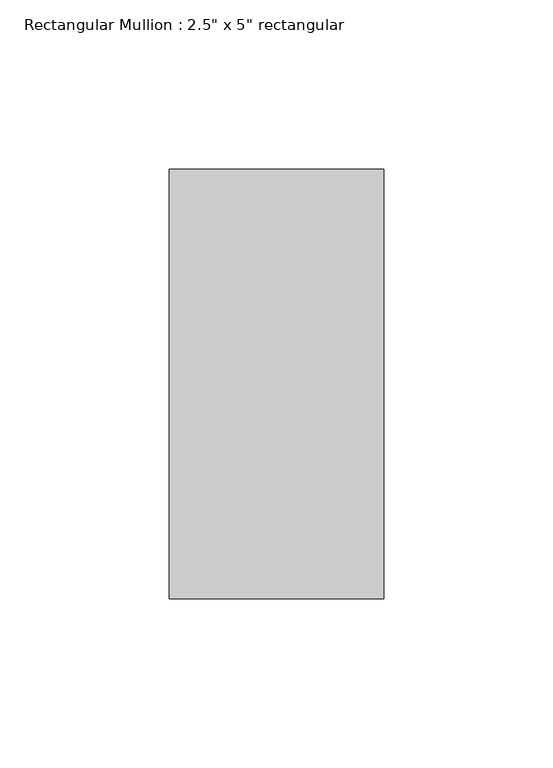
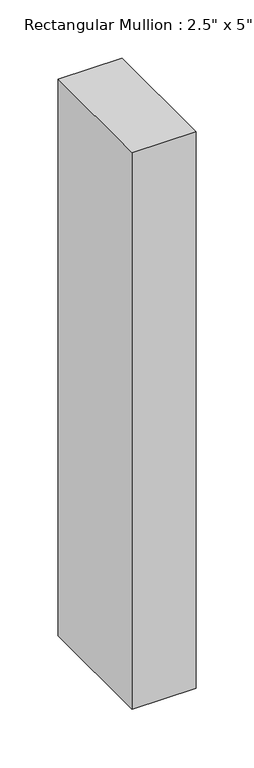
"""IFC4 building model written with IfcOpenShell, lengths in millimetres: member geometry."""

from ifc_helpers import new_model, si_unit, frame, origin, place, context, project, spatial, polyline, outline, extrude, source, transform, mapped, element, save


def member_2c0166dc(model_context):
    return source(origin(), model_context, "Body", "SweptSolid", [
        extrude(outline(polyline([(31.75, 63.5), (31.75, -63.5), (-31.75, -63.5), (-31.75, 63.5), (31.75, 63.5)])), frame((0.0, 0.0, -583.8967564), z_axis=(0.0, 0.0, 1.0), x_axis=(1.0, 0.0, 0.0)), (0.0, 0.0, 1.0), 583.8967564),
    ])


if __name__ == "__main__":
    model = new_model("IFC4")
    model_context = context("Model", 3, world=origin())
    ifc_project = project(units=[si_unit("LENGTHUNIT", "METRE", prefix="MILLI")], contexts=[model_context])
    site = spatial("IfcSite", under=ifc_project)
    building = spatial("IfcBuilding", under=site)
    placement = place(None, origin())
    member_shape = member_2c0166dc(model_context)
    element("IfcMember", 1, ObjectType="Rectangular Mullion : 2.5\" x 5\" rectangular", at=placement, inside=building, context=model_context, shape_type="MappedRepresentation", body=[
        mapped(member_shape, transform((0.0, 0.0, 0.0), x_axis=(1.0, 0.0, 0.0), y_axis=(0.0, 1.0, 0.0), z_axis=(0.0, 0.0, 1.0))),
    ])
    save(model, "model.ifc")

# Revit data of these elements
# Type "Rectangular Mullion : 2.5\" x 5\" rectangular"
#   built-in parameter 1007304 = 0.416667 (stored number, unit not read)
#   built-in parameter 1007301 = 0.104167 (stored number, unit not read)
#   built-in parameter 1007300 = 0.104167 (stored number, unit not read)
# Element 1 (IfcMember, "Rectangular Mullion : 2.5\" x 5\" rectangular")
#   Materials on its faces: "Aluminum"
# Materials
#   "Aluminum": class "Metal", colour RGB 247 247 247, transparency 0, Description = "Aluminum 6061", Cost = 0
